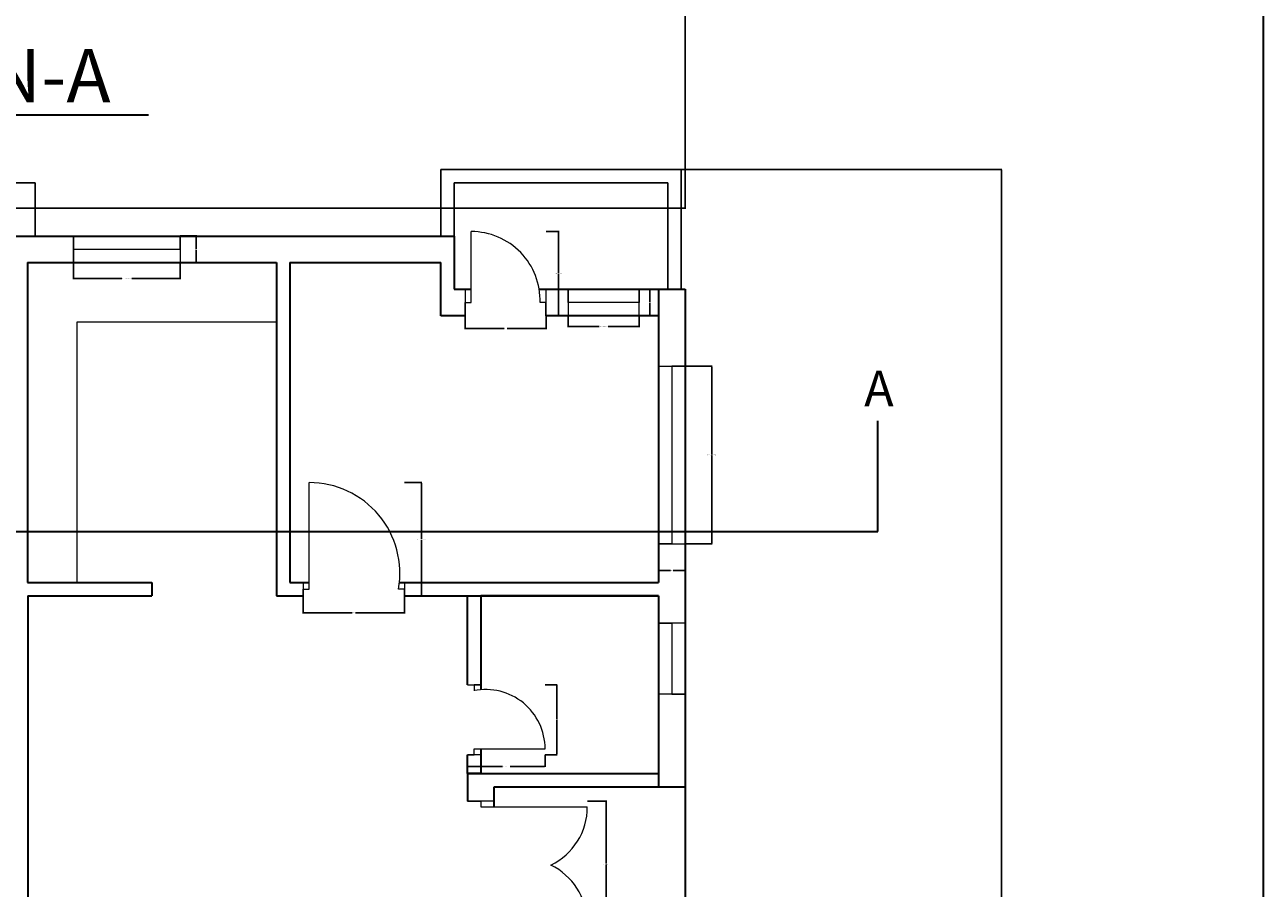
# Model space of a CAD drawing. Units: inches. Extents: x 2250 to 3629, y 982 to 2740.
# Tile 10 of 12: x 3211 to 3629, y 1828 to 2119. Entities that reach past the tile are written whole.
import ezdxf

# ---------------------------------------------------------------- set-up
doc = ezdxf.new("R2010")
doc.units = ezdxf.units.IN
for name, color, linetype, lineweight in [('A-ANNO-DIMS', 2, 'Continuous', 18), ('A-ANNO-SYMB', 7, 'Continuous', 35), ('A-ANNO-TITL', 7, 'Continuous', 35), ('A-ANNO-TTLB', 7, 'Continuous', 35), ('A-DOOR', 3, 'Continuous', 18), ('A-FLOR-DECK', 7, 'Continuous', 25), ('A-FLOR-FIXT', 9, 'Continuous', 18), ('A-GLAZ', 4, 'Continuous', 18), ('A-WALL', 7, 'Continuous', 35)]:
    doc.layers.add(name, color=color, linetype=linetype, lineweight=lineweight)
doc.styles.get("Standard").update_dxf_attribs({"font": 'arial.ttf'})
doc.dimstyles.get("Standard").update_dxf_attribs({"dimtxt": 0.18, "dimasz": 0.18, "dimexe": 0.18, "dimexo": 0.0625, "dimgap": 0.09, "dimtad": 0, "dimtih": 1, "dimtoh": 1, "dimdec": 4, "dimzin": 0, "dimdsep": 46, "dimtxsty": 'Standard', "dimcen": 0.09, "dimadec": 0, "dimazin": 0, "dimtfac": 1, "dimtdec": 4, "dimtofl": 0, "dimtmove": 0, "dimatfit": 3, "dimfxl": 1, "dimtolj": 1, "dimtzin": 0, "dimarcsym": 0})

# ---------------------------------------------------------------- blocks, each defined once
blk = doc.blocks.new('DR-36-BED-NE')
for p, q in [((2, 2.25), (2, 38.25)), ((0, 4.5), (0, 0)), ((34.14, 4.5), (34.14, 0)), ((0, 0), (0, 2.25)), ((0, 2.25), (2, 2.25)), ((34.14, 2.25), (32.14, 2.25)), ((34.14, 0), (34.14, 2.25))]:
    blk.add_line(p, q)
blk.add_arc((2, 7.63), 30.62, 349.8775, 90)
blk = doc.blocks.new('DR-24-DECK-NE')
for p, q in [((2, 4.5), (2, 28.5)), ((0, 9), (0, 0)), ((27.25, 9), (27.25, 0)), ((0, 0), (0, 4.5)), ((0, 4.5), (2, 4.5)), ((27.25, 4.5), (25.25, 4.5)), ((27.25, 0), (27.25, 4.5))]:
    blk.add_line(p, q)
blk.add_arc((2, 5.23), 23.27, 358.191, 90)
blk = doc.blocks.new('DR-24-BATH-NE')
for p, q in [((0, 23.65), (4.5, 23.65)), ((4.5, 23.65), (2.25, 23.65)), ((2.25, 23.65), (2.25, 21.65)), ((4.5, 0), (0, 0)), ((0, 0), (0, 0)), ((0, 0), (2.25, 0)), ((2.25, 0), (2.25, 2)), ((2.25, 2), (26.25, 2))]:
    blk.add_line(p, q)
blk.add_arc((6.2, 2), 20.05, 0, 101.3787)
blk = doc.blocks.new('DR-72-DECK-EAST-N')
for p, q in [((9, 42.6), (0, 42.6)), ((0, 42.6), (4.5, 42.6)), ((4.5, 42.6), (4.5, 40.6)), ((4.5, 40.6), (40.5, 40.6)), ((9, 0), (0, 0)), ((0, 0), (4.5, 0)), ((4.5, 0), (4.5, 2)), ((4.5, 2), (40.5, 2))]:
    blk.add_line(p, q)
for centre, radius, start, end in [((18.63, 40.6), 21.87, 295.9981, 0), ((18.59, 1.24), 21.93, 1.9829, 63.9515)]:
    blk.add_arc(centre, radius, start, end)
blk = doc.blocks.new('WIN-24-DECK-NE')
for p, q in [((0, 4.5), (0, 9)), ((0, 9), (0, 0)), ((24, 0), (24, 9)), ((24, 9), (24, 4.5)), ((24, 4.5), (0, 4.5))]:
    blk.add_line(p, q)
blk = doc.blocks.new('WIN-60-BED-NE')
for p, q in [((0, 60), (9, 60)), ((9, 60), (4.5, 60)), ((4.5, 60), (4.5, 12)), ((4.5, 12), (4.5, 0)), ((4.5, 0), (0, 0)), ((0, 0), (9, 0))]:
    blk.add_line(p, q)
blk = doc.blocks.new('WIN-36-KITCHEN-NE')
for p, q in [((0, 9), (0, 0)), ((0, 0), (0, 9)), ((0, 9), (0, 4.5)), ((36, 4.5), (36, 9)), ((36, 9), (36, 0)), ((0, 4.5), (36, 4.5))]:
    blk.add_line(p, q)
blk = doc.blocks.new('WIN-24-BATH-NW')
for p, q in [((9, 24), (0, 24)), ((0, 24), (4.5, 24)), ((4.5, 24), (4.5, 0)), ((9, 0), (0, 0)), ((4.5, 0), (9, 0))]:
    blk.add_line(p, q)
blk = doc.blocks.new('*D75')
at = {"layer": 'A-ANNO-DIMS', "color": 0, "lineweight": -2, "transparency": 16777216}
for p, q in [((3394.77, 2020.67), (3394.77, 2016.96)), ((3418.77, 2020.67), (3418.77, 2016.96)), ((3394.95, 2017.14), (3405.28, 2017.14)), ((3418.59, 2017.14), (3408.27, 2017.14))]:
    blk.add_line(p, q, dxfattribs=at)
at = {"layer": 'A-ANNO-DIMS', "color": 0, "transparency": 16777216}
for points in [[(3394.95, 2017.17), (3394.95, 2017.11), (3394.77, 2017.14)], [(3418.59, 2017.17), (3418.59, 2017.11), (3418.77, 2017.14)]]:
    blk.add_solid(points, dxfattribs=at)
at = {"layer": 'Defpoints', "color": 0, "transparency": 16777216}
for p in [(3394.77, 2020.74), (3418.77, 2020.74), (3418.77, 2017.14)]:
    blk.add_point(p, dxfattribs=at)
at = {"layer": 'A-ANNO-DIMS', "color": 0, "transparency": 16777216, "insert": (3406.77, 2017.14), "char_height": 0.18, "attachment_point": 5}
blk.add_mtext('\\A1;DECK WINDOW 24 TYP.', dxfattribs=at)
blk = doc.blocks.new('*D76')
at = {"layer": 'A-ANNO-DIMS', "color": 0, "lineweight": -2, "transparency": 16777216}
for p, q in [((3418.84, 2029.74), (3422.55, 2029.74)), ((3422.37, 2029.56), (3422.37, 2025.42)), ((3422.37, 2020.92), (3422.37, 2025.05)), ((3418.84, 2020.74), (3422.55, 2020.74))]:
    blk.add_line(p, q, dxfattribs=at)
at = {"layer": 'A-ANNO-DIMS', "color": 0, "transparency": 16777216}
for points in [[(3422.34, 2029.56), (3422.4, 2029.56), (3422.37, 2029.74)], [(3422.34, 2020.92), (3422.4, 2020.92), (3422.37, 2020.74)]]:
    blk.add_solid(points, dxfattribs=at)
at = {"layer": 'Defpoints', "color": 0, "transparency": 16777216}
for p in [(3418.77, 2029.74), (3422.37, 2029.74), (3418.77, 2020.74)]:
    blk.add_point(p, dxfattribs=at)
at = {"layer": 'A-ANNO-DIMS', "color": 0, "transparency": 16777216, "insert": (3422.37, 2025.24), "char_height": 0.18, "attachment_point": 5}
blk.add_mtext('\\A1;9 TYP.', dxfattribs=at)
blk = doc.blocks.new('*D77')
at = {"layer": 'A-ANNO-DIMS', "color": 0, "lineweight": -2, "transparency": 16777216}
for p, q in [((3227.74, 2038.67), (3227.74, 2033.16)), ((3263.74, 2038.67), (3263.74, 2033.16)), ((3227.92, 2033.34), (3244.04, 2033.34)), ((3263.56, 2033.34), (3247.43, 2033.34))]:
    blk.add_line(p, q, dxfattribs=at)
at = {"layer": 'A-ANNO-DIMS', "color": 0, "transparency": 16777216}
for points in [[(3227.92, 2033.37), (3227.92, 2033.31), (3227.74, 2033.34)], [(3263.56, 2033.37), (3263.56, 2033.31), (3263.74, 2033.34)]]:
    blk.add_solid(points, dxfattribs=at)
at = {"layer": 'Defpoints', "color": 0, "transparency": 16777216}
for p in [(3227.74, 2038.74), (3263.74, 2038.74), (3263.74, 2033.34)]:
    blk.add_point(p, dxfattribs=at)
at = {"layer": 'A-ANNO-DIMS', "color": 0, "transparency": 16777216, "insert": (3245.74, 2033.34), "char_height": 0.18, "attachment_point": 5}
blk.add_mtext('\\A1;KITCHEN WINDOW 36 TYP.', dxfattribs=at)
blk = doc.blocks.new('*D78')
at = {"layer": 'A-ANNO-DIMS', "color": 0, "lineweight": -2, "transparency": 16777216}
for p, q in [((3263.8, 2047.74), (3269.32, 2047.74)), ((3269.14, 2047.56), (3269.14, 2043.42)), ((3269.14, 2038.92), (3269.14, 2043.05)), ((3263.8, 2038.74), (3269.32, 2038.74))]:
    blk.add_line(p, q, dxfattribs=at)
at = {"layer": 'A-ANNO-DIMS', "color": 0, "transparency": 16777216}
for points in [[(3269.11, 2047.56), (3269.17, 2047.56), (3269.14, 2047.74)], [(3269.11, 2038.92), (3269.17, 2038.92), (3269.14, 2038.74)]]:
    blk.add_solid(points, dxfattribs=at)
at = {"layer": 'Defpoints', "color": 0, "transparency": 16777216}
for p in [(3263.74, 2047.74), (3269.14, 2047.74), (3263.74, 2038.74)]:
    blk.add_point(p, dxfattribs=at)
at = {"layer": 'A-ANNO-DIMS', "color": 0, "transparency": 16777216, "insert": (3269.14, 2043.24), "char_height": 0.18, "attachment_point": 5}
blk.add_mtext('\\A1;9 TYP.', dxfattribs=at)
blk = doc.blocks.new('*D83')
at = {"layer": 'A-ANNO-DIMS', "color": 0, "lineweight": -2, "transparency": 16777216}
for p, q in [((3434.29, 2003.78), (3443.41, 2003.78)), ((3443.23, 2003.6), (3443.23, 1973.96)), ((3443.23, 1943.96), (3443.23, 1973.6)), ((3434.29, 1943.78), (3443.41, 1943.78))]:
    blk.add_line(p, q, dxfattribs=at)
at = {"layer": 'A-ANNO-DIMS', "color": 0, "transparency": 16777216}
for points in [[(3443.2, 2003.6), (3443.26, 2003.6), (3443.23, 2003.78)], [(3443.2, 1943.96), (3443.26, 1943.96), (3443.23, 1943.78)]]:
    blk.add_solid(points, dxfattribs=at)
at = {"layer": 'Defpoints', "color": 0, "transparency": 16777216}
for p in [(3434.23, 2003.78), (3443.23, 2003.78), (3434.23, 1943.78)]:
    blk.add_point(p, dxfattribs=at)
at = {"layer": 'A-ANNO-DIMS', "color": 0, "transparency": 16777216, "insert": (3443.23, 1973.78), "char_height": 0.18, "attachment_point": 5}
blk.add_mtext('\\A1;BEDROOM WINDOW 60 TYP.', dxfattribs=at)
blk = doc.blocks.new('*D84')
at = {"layer": 'A-ANNO-DIMS', "color": 0, "lineweight": -2, "transparency": 16777216}
for p, q in [((3425.23, 1943.72), (3425.23, 1934.6)), ((3434.23, 1943.72), (3434.23, 1934.6)), ((3425.41, 1934.78), (3429.27, 1934.78)), ((3434.05, 1934.78), (3430.18, 1934.78))]:
    blk.add_line(p, q, dxfattribs=at)
at = {"layer": 'A-ANNO-DIMS', "color": 0, "transparency": 16777216}
for points in [[(3425.41, 1934.81), (3425.41, 1934.75), (3425.23, 1934.78)], [(3434.05, 1934.81), (3434.05, 1934.75), (3434.23, 1934.78)]]:
    blk.add_solid(points, dxfattribs=at)
at = {"layer": 'Defpoints', "color": 0, "transparency": 16777216}
for p in [(3425.23, 1943.78), (3434.23, 1943.78), (3434.23, 1934.78)]:
    blk.add_point(p, dxfattribs=at)
at = {"layer": 'A-ANNO-DIMS', "color": 0, "transparency": 16777216, "insert": (3429.73, 1934.78), "char_height": 0.18, "attachment_point": 5}
blk.add_mtext('\\A1;9 TYP.', dxfattribs=at)
blk = doc.blocks.new('*D99')
at = {"layer": 'A-ANNO-DIMS', "color": 0, "lineweight": -2, "transparency": 16777216}
for p, q in [((3339.53, 1964.49), (3345.39, 1964.49)), ((3345.21, 1964.31), (3345.21, 1945.54)), ((3345.21, 1926.42), (3345.21, 1945.18)), ((3339.53, 1926.24), (3345.39, 1926.24))]:
    blk.add_line(p, q, dxfattribs=at)
at = {"layer": 'A-ANNO-DIMS', "color": 0, "transparency": 16777216}
for points in [[(3345.18, 1964.31), (3345.24, 1964.31), (3345.21, 1964.49)], [(3345.18, 1926.42), (3345.24, 1926.42), (3345.21, 1926.24)]]:
    blk.add_solid(points, dxfattribs=at)
at = {"layer": 'Defpoints', "color": 0, "transparency": 16777216}
for p in [(3339.47, 1964.49), (3345.21, 1964.49), (3339.47, 1926.24)]:
    blk.add_point(p, dxfattribs=at)
at = {"layer": 'A-ANNO-DIMS', "color": 0, "transparency": 16777216, "insert": (3345.21, 1945.36), "char_height": 0.18, "attachment_point": 5}
blk.add_mtext('\\A1;BEDROOM DOOR 38 TYP.', dxfattribs=at)
blk = doc.blocks.new('*D100')
at = {"layer": 'A-ANNO-DIMS', "color": 0, "lineweight": -2, "transparency": 16777216}
for p, q in [((3305.33, 1926.17), (3305.33, 1920.32)), ((3339.47, 1926.17), (3339.47, 1920.32)), ((3305.51, 1920.5), (3321.87, 1920.5)), ((3339.29, 1920.5), (3322.93, 1920.5))]:
    blk.add_line(p, q, dxfattribs=at)
at = {"layer": 'A-ANNO-DIMS', "color": 0, "transparency": 16777216}
for points in [[(3305.51, 1920.53), (3305.51, 1920.47), (3305.33, 1920.5)], [(3339.29, 1920.53), (3339.29, 1920.47), (3339.47, 1920.5)]]:
    blk.add_solid(points, dxfattribs=at)
at = {"layer": 'Defpoints', "color": 0, "transparency": 16777216}
for p in [(3305.33, 1926.24), (3339.47, 1926.24), (3339.47, 1920.5)]:
    blk.add_point(p, dxfattribs=at)
at = {"layer": 'A-ANNO-DIMS', "color": 0, "transparency": 16777216, "insert": (3322.4, 1920.5), "char_height": 0.18, "attachment_point": 5}
blk.add_mtext('\\A1;34 TYP.', dxfattribs=at)
blk = doc.blocks.new('*D101')
at = {"layer": 'A-ANNO-DIMS', "color": 0, "lineweight": -2, "transparency": 16777216}
for p, q in [((3387.34, 2049.24), (3391.73, 2049.24)), ((3391.55, 2049.06), (3391.55, 2035.17)), ((3391.55, 2020.92), (3391.55, 2034.8)), ((3387.34, 2020.74), (3391.73, 2020.74))]:
    blk.add_line(p, q, dxfattribs=at)
at = {"layer": 'A-ANNO-DIMS', "color": 0, "transparency": 16777216}
for points in [[(3391.52, 2049.06), (3391.58, 2049.06), (3391.55, 2049.24)], [(3391.52, 2020.92), (3391.58, 2020.92), (3391.55, 2020.74)]]:
    blk.add_solid(points, dxfattribs=at)
at = {"layer": 'Defpoints', "color": 0, "transparency": 16777216}
for p in [(3387.28, 2049.24), (3391.55, 2049.24), (3387.28, 2020.74)]:
    blk.add_point(p, dxfattribs=at)
at = {"layer": 'A-ANNO-DIMS', "color": 0, "transparency": 16777216, "insert": (3391.55, 2034.99), "char_height": 0.18, "attachment_point": 5}
blk.add_mtext('\\A1;DECK DOOR 29 TYP.', dxfattribs=at)
blk = doc.blocks.new('*D102')
at = {"layer": 'A-ANNO-DIMS', "color": 0, "lineweight": -2, "transparency": 16777216}
for p, q in [((3360.02, 2020.67), (3360.02, 2016.28)), ((3387.28, 2020.67), (3387.28, 2016.28)), ((3360.2, 2016.46), (3373.12, 2016.46)), ((3387.1, 2016.46), (3374.18, 2016.46))]:
    blk.add_line(p, q, dxfattribs=at)
at = {"layer": 'A-ANNO-DIMS', "color": 0, "transparency": 16777216}
for points in [[(3360.2, 2016.49), (3360.2, 2016.43), (3360.02, 2016.46)], [(3387.1, 2016.49), (3387.1, 2016.43), (3387.28, 2016.46)]]:
    blk.add_solid(points, dxfattribs=at)
at = {"layer": 'Defpoints', "color": 0, "transparency": 16777216}
for p in [(3360.02, 2020.74), (3387.28, 2020.74), (3387.28, 2016.46)]:
    blk.add_point(p, dxfattribs=at)
at = {"layer": 'A-ANNO-DIMS', "color": 0, "transparency": 16777216, "insert": (3373.65, 2016.46), "char_height": 0.18, "attachment_point": 5}
blk.add_mtext('\\A1;27 TYP.', dxfattribs=at)
blk = doc.blocks.new('*D111')
at = {"layer": 'A-ANNO-DIMS', "color": 0, "lineweight": -2, "transparency": 16777216}
for p, q in [((3360.73, 1872.52), (3360.73, 1868.47)), ((3386.98, 1872.52), (3386.98, 1868.47)), ((3360.91, 1868.65), (3372.55, 1868.65)), ((3386.8, 1868.65), (3375.16, 1868.65))]:
    blk.add_line(p, q, dxfattribs=at)
at = {"layer": 'A-ANNO-DIMS', "color": 0, "transparency": 16777216}
for points in [[(3360.91, 1868.68), (3360.91, 1868.62), (3360.73, 1868.65)], [(3386.8, 1868.68), (3386.8, 1868.62), (3386.98, 1868.65)]]:
    blk.add_solid(points, dxfattribs=at)
at = {"layer": 'Defpoints', "color": 0, "transparency": 16777216}
for p in [(3360.73, 1872.58), (3386.98, 1872.58), (3386.98, 1868.65)]:
    blk.add_point(p, dxfattribs=at)
at = {"layer": 'A-ANNO-DIMS', "color": 0, "transparency": 16777216, "insert": (3373.85, 1868.65), "char_height": 0.18, "attachment_point": 5}
blk.add_mtext('\\A1;BATH DOOR 26 TYP.', dxfattribs=at)
blk = doc.blocks.new('*D112')
at = {"layer": 'A-ANNO-DIMS', "color": 0, "lineweight": -2, "transparency": 16777216}
for p, q in [((3387.04, 1896.24), (3391.09, 1896.24)), ((3390.91, 1896.06), (3390.91, 1884.59)), ((3390.91, 1872.76), (3390.91, 1884.23)), ((3387.04, 1872.58), (3391.09, 1872.58))]:
    blk.add_line(p, q, dxfattribs=at)
at = {"layer": 'A-ANNO-DIMS', "color": 0, "transparency": 16777216}
for points in [[(3390.88, 1896.06), (3390.94, 1896.06), (3390.91, 1896.24)], [(3390.88, 1872.76), (3390.94, 1872.76), (3390.91, 1872.58)]]:
    blk.add_solid(points, dxfattribs=at)
at = {"layer": 'Defpoints', "color": 0, "transparency": 16777216}
for p in [(3386.98, 1896.24), (3390.91, 1896.24), (3386.98, 1872.58)]:
    blk.add_point(p, dxfattribs=at)
at = {"layer": 'A-ANNO-DIMS', "color": 0, "transparency": 16777216, "insert": (3390.91, 1884.41), "char_height": 0.18, "attachment_point": 5}
blk.add_mtext('\\A1;24 TYP.', dxfattribs=at)
blk = doc.blocks.new('*D115')
at = {"layer": 'A-ANNO-DIMS', "color": 0, "lineweight": -2, "transparency": 16777216}
for p, q in [((3401.29, 1856.98), (3407.8, 1856.98)), ((3407.62, 1856.8), (3407.62, 1835.86)), ((3407.62, 1814.56), (3407.62, 1835.5)), ((3401.29, 1814.38), (3407.8, 1814.38))]:
    blk.add_line(p, q, dxfattribs=at)
at = {"layer": 'A-ANNO-DIMS', "color": 0, "transparency": 16777216}
for points in [[(3407.59, 1856.8), (3407.65, 1856.8), (3407.62, 1856.98)], [(3407.59, 1814.56), (3407.65, 1814.56), (3407.62, 1814.38)]]:
    blk.add_solid(points, dxfattribs=at)
at = {"layer": 'Defpoints', "color": 0, "transparency": 16777216}
for p in [(3401.23, 1856.98), (3407.62, 1856.98), (3401.23, 1814.38)]:
    blk.add_point(p, dxfattribs=at)
at = {"layer": 'A-ANNO-DIMS', "color": 0, "transparency": 16777216, "insert": (3407.62, 1835.68), "char_height": 0.18, "attachment_point": 5}
blk.add_mtext('\\A1;DECK DOOR 43 TYP.', dxfattribs=at)
blk = doc.blocks.new('*D172')
at = {"layer": 'A-ANNO-DIMS', "color": 0, "lineweight": -2, "transparency": 16777216}
for p, q in [((3433.02, 2070.24), (3541.21, 2070.24)), ((3541.03, 2070.06), (3541.03, 1664.67)), ((3541.03, 1258.92), (3541.03, 1664.3)), ((3059.29, 1258.74), (3541.21, 1258.74))]:
    blk.add_line(p, q, dxfattribs=at)
at = {"layer": 'A-ANNO-DIMS', "color": 0, "transparency": 16777216}
for points in [[(3541, 2070.06), (3541.06, 2070.06), (3541.03, 2070.24)], [(3541, 1258.92), (3541.06, 1258.92), (3541.03, 1258.74)]]:
    blk.add_solid(points, dxfattribs=at)
at = {"layer": 'Defpoints', "color": 0, "transparency": 16777216}
for p in [(3432.96, 2070.24), (3541.03, 2070.24), (3059.23, 1258.74)]:
    blk.add_point(p, dxfattribs=at)
at = {"layer": 'A-ANNO-DIMS', "color": 0, "transparency": 16777216, "insert": (3541.03, 1664.49), "char_height": 0.18, "attachment_point": 5}
blk.add_mtext('\\A1;811.5', dxfattribs=at)
blk = doc.blocks.new('*D188')
at = {"layer": 'A-ANNO-DIMS', "color": 0, "lineweight": -2, "transparency": 16777216}
for p, q in [((2981.23, 2131.64), (2981.23, 2056.9)), ((3434.23, 2131.64), (3434.23, 2056.9)), ((2981.41, 2057.08), (3207.43, 2057.08)), ((3434.05, 2057.08), (3208.02, 2057.08))]:
    blk.add_line(p, q, dxfattribs=at)
at = {"layer": 'A-ANNO-DIMS', "color": 0, "transparency": 16777216}
for points in [[(2981.41, 2057.11), (2981.41, 2057.05), (2981.23, 2057.08)], [(3434.05, 2057.11), (3434.05, 2057.05), (3434.23, 2057.08)]]:
    blk.add_solid(points, dxfattribs=at)
at = {"layer": 'Defpoints', "color": 0, "transparency": 16777216}
for p in [(2981.23, 2131.7), (3434.23, 2131.7), (3434.23, 2057.08)]:
    blk.add_point(p, dxfattribs=at)
at = {"layer": 'A-ANNO-DIMS', "color": 0, "transparency": 16777216, "insert": (3207.73, 2057.08), "char_height": 0.18, "attachment_point": 5}
blk.add_mtext('\\A1;453', dxfattribs=at)

msp = doc.modelspace()

# ---------------------------------------------------------------- linework, layer by layer
at = {"layer": 'A-ANNO-SYMB'}
for p, q in [((3499.2778, 1947.9231), (3499.2778, 1985.3261)), ((2932.0741, 1947.9231), (3499.2778, 1947.9231))]:
    msp.add_line(p, q, dxfattribs=at)
at = {"layer": 'A-ANNO-TITL'}
msp.add_line((3253.0344, 2088.5817), (3106.2899, 2088.5817), dxfattribs=at)
at = {"layer": 'A-ANNO-TTLB'}
msp.add_lwpolyline([(2249.6849, 2739.593), (3629.4532, 2739.593), (3629.4532, 982.3108), (2249.6849, 982.3108)], close=True, dxfattribs=at)
at = {"layer": 'A-FLOR-DECK'}
for p, q in [((3432.9579, 2070.2354), (3351.7267, 2070.2354)), ((3351.7267, 2070.2354), (3351.7267, 2047.7354)), ((3432.9579, 2065.7354), (3432.9579, 2070.2354)), ((3139.754, 2065.7354), (3214.8276, 2065.7354)), ((3214.8276, 2065.7354), (3214.8276, 2047.7354)), ((3356.2267, 2047.7354), (3356.2267, 2065.7354)), ((3356.2267, 2065.7354), (3428.4579, 2065.7354)), ((3428.4579, 2065.7354), (3428.4579, 2029.7354)), ((3432.9579, 2029.7354), (3432.9579, 2065.7354)), ((3214.8276, 2047.7354), (3210.3276, 2047.7354))]:
    msp.add_line(p, q, dxfattribs=at)
at = {"layer": 'A-FLOR-FIXT'}
for p, q in [((3229.015, 1930.7354), (3229.015, 2018.7457)), ((3229.015, 2018.7457), (3296.2267, 2018.7457))]:
    msp.add_line(p, q, dxfattribs=at)
at = {"layer": 'A-WALL'}
for p, q in [((3203.2267, 2047.7354), (3356.2267, 2047.7354)), ((3356.2267, 2047.7354), (3356.2267, 2029.7354)), ((3212.2267, 2038.7354), (3212.2267, 1930.7354)), ((3212.2267, 2038.7354), (3296.2267, 2038.7354)), ((3296.2267, 2038.7354), (3296.2267, 1930.7354)), ((3300.7267, 2038.7354), (3300.7267, 1930.7354)), ((3300.7267, 2038.7354), (3351.7267, 2038.7354)), ((3351.7267, 2020.7354), (3351.7267, 2038.7354)), ((3356.2267, 2029.7354), (3362.0215, 2029.7354)), ((3384.9803, 2029.7354), (3425.2267, 2029.7354)), ((3425.2267, 2029.7354), (3425.2267, 1930.7354)), ((3425.2267, 2029.7354), (3425.2267, 2020.7354)), ((3425.2267, 2029.7354), (3434.2267, 2029.7354)), ((3434.2267, 2029.7354), (3434.2267, 1276.7354)), ((3356.2267, 2020.7354), (3351.7267, 2020.7354)), ((3360.0215, 2020.7354), (3356.2267, 2020.7354)), ((3425.2267, 2020.7354), (3387.2755, 2020.7354)), ((3212.2267, 1930.7354), (3254.2267, 1930.7354)), ((3254.2267, 1930.7354), (3254.2267, 1926.2354)), ((3296.2267, 1930.7354), (3296.2267, 1926.2354)), ((3300.7267, 1930.7354), (3307.3283, 1930.7354)), ((3337.7864, 1930.7354), (3425.2267, 1930.7354)), ((3212.321, 1926.2354), (3254.2267, 1926.2354)), ((3212.321, 1926.2354), (3212.321, 1789.7354)), ((3296.2267, 1926.2354), (3305.3283, 1926.2354)), ((3339.4703, 1926.2354), (3425.2267, 1926.2354)), ((3360.7267, 1896.2354), (3360.7267, 1926.2354)), ((3425.2267, 1926.2354), (3365.2267, 1926.2354)), ((3365.2267, 1926.2354), (3365.2267, 1894.5568)), ((3425.2267, 1926.2354), (3425.2267, 1861.7354)), ((3365.2267, 1874.5842), (3365.2267, 1866.2354)), ((3360.7267, 1866.2354), (3360.7267, 1872.5842)), ((3360.7267, 1866.2354), (3425.2267, 1866.2354)), ((3365.2267, 1866.2354), (3360.7267, 1866.2354)), ((3360.7267, 1866.2354), (3360.7267, 1856.9787)), ((3369.7267, 1861.7354), (3434.2267, 1861.7354)), ((3369.7267, 1854.9787), (3369.7267, 1861.7354))]:
    msp.add_line(p, q, dxfattribs=at)

# ---------------------------------------------------------------- block references
at = {"layer": 'A-DOOR'}
for name, p in [('DR-24-DECK-NE', (3360.0215, 2020.735)), ('DR-36-BED-NE', (3305.3285, 1926.235)), ('DR-24-BATH-NE', (3360.7265, 1872.584)), ('DR-72-DECK-EAST-N', (3360.7265, 1814.38))]:
    msp.add_blockref(name, p, dxfattribs=at)
at = {"layer": 'A-GLAZ'}
for name, p in [('WIN-36-KITCHEN-NE', (3227.7375, 2038.735)), ('WIN-24-DECK-NE', (3394.7725, 2020.735)), ('WIN-60-BED-NE', (3425.2265, 1943.78)), ('WIN-24-BATH-NW', (3425.2265, 1893.0165))]:
    msp.add_blockref(name, p, dxfattribs=at)

# ---------------------------------------------------------------- texts
at = {"layer": 'A-ANNO-SYMB', "insert": (3494.7142, 2002.2191), "char_height": 12, "attachment_point": 1}
msp.add_mtext_dynamic_manual_height_columns('A', width=12.825745, gutter_width=12.5, heights=[0], dxfattribs=at)
at = {"layer": 'A-ANNO-TITL', "insert": (3114.1642, 2110.8168), "char_height": 18, "attachment_point": 1}
msp.add_mtext_dynamic_manual_height_columns('SECTION-A', width=241.677358, gutter_width=12.5, heights=[0], dxfattribs=at)

# ---------------------------------------------------------------- dimensions: what is measured, and where the dimension line sits
at = {"layer": 'A-ANNO-DIMS'}
dim = msp.add_linear_dim(base=(3434.2267, 2057.0817), p1=(2981.2267, 2131.6999), p2=(3434.2267, 2131.6999), dimstyle='Standard', override={"dimdec": 0, "dimlfac": 1, "dimrnd": 0, "dimzin": 0, "dimdsep": 46, "dimlunit": 2}, dxfattribs=at)
dim.commit()
dim.dimension.update_dxf_attribs({"geometry": '*D188', "text_midpoint": (3207.7267, 2057.0817)})
dim = msp.add_linear_dim(base=(3541.0278, 2070.2354), p1=(3059.2267, 1258.7354), p2=(3432.9579, 2070.2354), angle=90, dimstyle='Standard', override={"dimdec": 1, "dimlfac": 1, "dimrnd": 0, "dimzin": 0, "dimdsep": 46, "dimlunit": 2}, dxfattribs=at)
dim.commit()
dim.dimension.update_dxf_attribs({"geometry": '*D172', "text_midpoint": (3541.0278, 1664.4854)})
for base, p1, p2, text, picture, middle in [((3391.5505049679, 2049.2354249075), (3387.2755049679, 2020.7354249075), (3387.2755049679, 2049.2354249075), 'DECK DOOR <> TYP.', '*D101', (3391.5505049679, 2034.9854249075)), ((3269.1374, 2047.7354), (3263.7374, 2038.7354), (3263.7374, 2047.7354), '<> TYP.', '*D78', (3269.1374, 2043.2354)), ((3422.3725, 2029.7354), (3418.7725, 2020.7354), (3418.7725, 2029.7354), '<> TYP.', '*D76', (3422.3725, 2025.2354)), ((3443.2267, 2003.7795), (3434.2267, 1943.7795), (3434.2267, 2003.7795), 'BEDROOM WINDOW <> TYP.', '*D83', (3443.2267, 1973.7795)), ((3345.2078, 1964.4854), (3339.4703, 1926.2354), (3339.4703, 1964.4854), 'BEDROOM DOOR <> TYP.', '*D99', (3345.2078, 1945.3604)), ((3390.9142, 1896.2354), (3386.9767, 1872.5842), (3386.9767, 1896.2354), '<> TYP.', '*D112', (3390.9142, 1884.4098)), ((3407.6165, 1856.9787), (3401.2267, 1814.3801), (3401.2267, 1856.9787), 'DECK DOOR <> TYP.', '*D115', (3407.6165, 1835.6794))]:
    dim = msp.add_linear_dim(base=base, p1=p1, p2=p2, angle=90, text=text, dimstyle='Standard', override={"dimdec": 0, "dimlfac": 1, "dimrnd": 0, "dimzin": 0, "dimdsep": 46, "dimlunit": 2}, dxfattribs=at)
    dim.commit()
    dim.dimension.update_dxf_attribs({"geometry": picture, "text_midpoint": middle})
for base, p1, p2, text, picture, middle in [((3263.7374, 2033.3354), (3227.7374, 2038.7354), (3263.7374, 2038.7354), 'KITCHEN WINDOW <> TYP.', '*D77', (3245.7374, 2033.3354)), ((3387.2755, 2016.4604), (3360.0215, 2020.7354), (3387.2755, 2020.7354), '<> TYP.', '*D102', (3373.6485, 2016.4604)), ((3418.7725, 2017.1354), (3394.7725, 2020.7354), (3418.7725, 2020.7354), 'DECK WINDOW <> TYP.', '*D75', (3406.7725, 2017.1354)), ((3434.2267, 1934.7795), (3425.2267, 1943.7795), (3434.2267, 1943.7795), '<> TYP.', '*D84', (3429.7267, 1934.7795)), ((3339.4703, 1920.4979), (3305.3283, 1926.2354), (3339.4703, 1926.2354), '<> TYP.', '*D100', (3322.3993, 1920.4979)), ((3386.9767, 1868.6467), (3360.7267, 1872.5842), (3386.9767, 1872.5842), 'BATH DOOR <> TYP.', '*D111', (3373.8517, 1868.6467))]:
    dim = msp.add_linear_dim(base=base, p1=p1, p2=p2, text=text, dimstyle='Standard', override={"dimdec": 0, "dimlfac": 1, "dimrnd": 0, "dimzin": 0, "dimdsep": 46, "dimlunit": 2}, dxfattribs=at)
    dim.commit()
    dim.dimension.update_dxf_attribs({"geometry": picture, "text_midpoint": middle})

doc.saveas('drawing.dxf')
